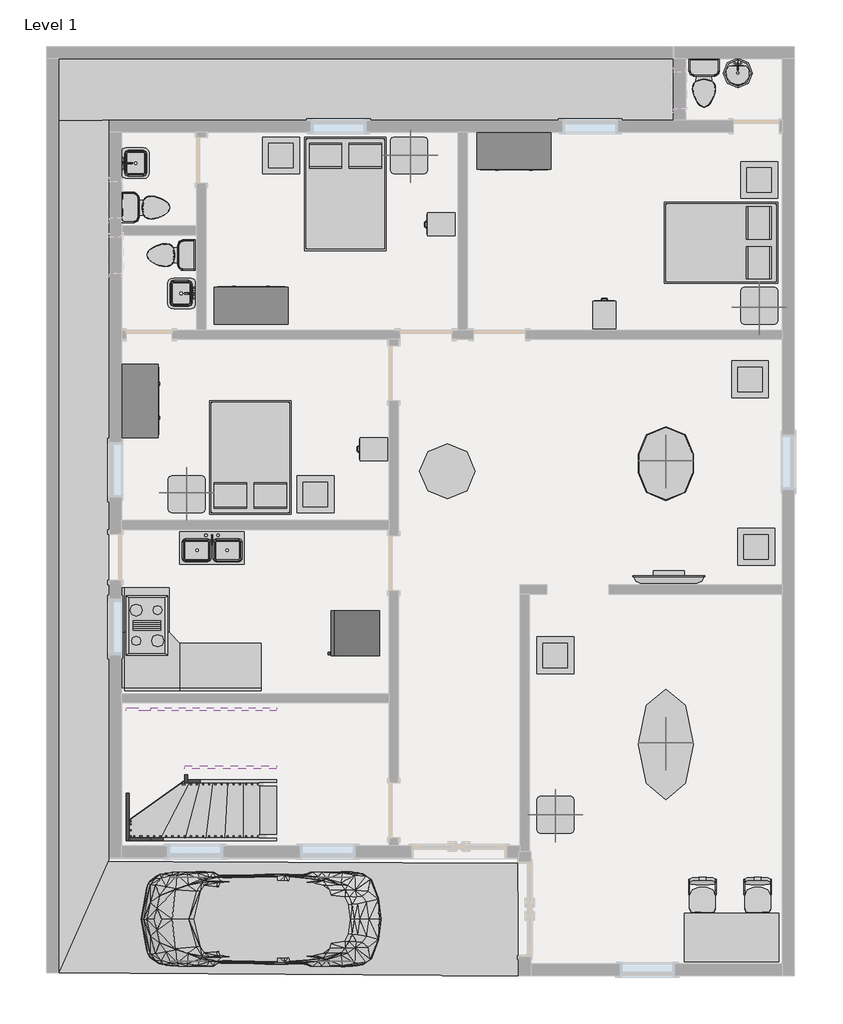
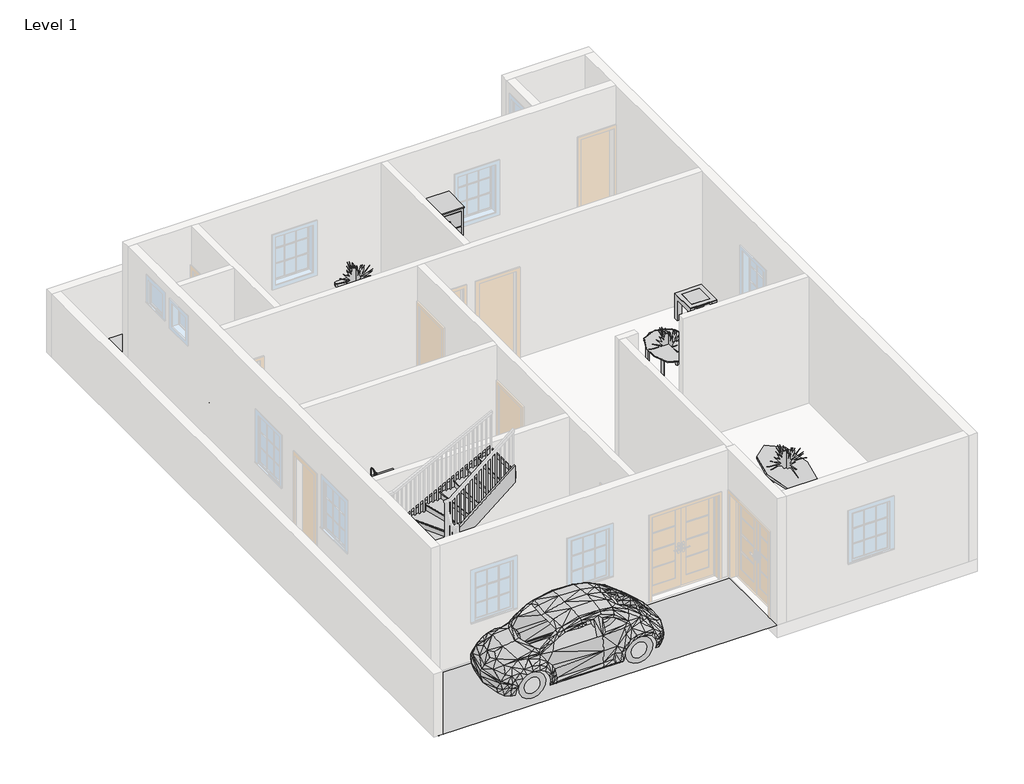
# One storey, part 3 of 3: 27 furniture elements, 10 flow terminals, 8 members, 6 geographic elements, 6 proxies, 1 stair flight.
"""IFC4 building model written with IfcOpenShell, lengths in millimetres."""

from ifc_helpers import new_model, si_unit, frame, origin, place, context, project, spatial, polyline, outline, extrude, triangles, transform, mapped, element, save
from components import proxy_bb1e6e30, rpc_beetle_rpc_beetle_3ce7ba48, proxy_a13a33b2, flow_terminal_accce45a, flow_terminal_a53be723, flow_terminal_d49f872f, flow_terminal_62a433f7, toilet_domestic_3d_toilet_domestic_3d_f7549cf7, toilet_domestic_3d_toilet_domestic_3d_183bbd19, furniture_c8abb964, furniture_bb55ed6b, furniture_072f6425, furniture_9fa109b2, furniture_3d1d9cbc, furniture_d9bcc661, furniture_b5c51a22, furniture_be1c6672, furniture_905aceb5, furniture_c0716227, furniture_31d08a24, furniture_cb58875c, rpc_plant_tropical_agave_1_5_93a2a214, stair_flight_2afbddc8

model = new_model("IFC4")

# Units and contexts
model_context = context("Model", 3, world=origin())
ifc_project = project(units=[si_unit("LENGTHUNIT", "METRE", prefix="MILLI")], contexts=[model_context])

# Site, building, storey
site = spatial("IfcSite", under=ifc_project)
building = spatial("IfcBuilding", under=site)
storey = spatial("IfcBuildingStorey", under=building, Name="Level 1", Elevation=0.0)

# Proxies
placement = place(None, origin())
element("IfcBuildingElementProxy", 1, Name="Building Element Proxy", at=placement, inside=storey, context=model_context, shape_type="Tessellation", body=[
    triangles([(813.744298, 15274.0246674, 0.0), (801.0442738, 14258.0250549, 0.0), (-9384.3556778, 14243.023645, 0.0), (-9384.3556778, 15274.0246674, 0.0)], [[4, 3, 2], [2, 1, 4]], closed=False),
])
element("IfcBuildingElementProxy", 2, Name="Building Element Proxy", at=placement, inside=storey, context=model_context, shape_type="Tessellation", body=[
    triangles([(-8546.1556778, 14258.0250549, 0.0), (-9384.3556778, 14196.8846008, 0.0), (-9384.3556778, 135.6245977, 0.0), (-9384.3556778, 2055.4156734, 0.0), (-8546.1556778, 2021.5745705, 0.0), (-9384.3556778, 14248.2919281, 0.0)], [[5, 4, 3], [5, 2, 4], [6, 2, 1], [5, 1, 2]], closed=False),
])
element("IfcBuildingElementProxy", 3, Name="Building Element Proxy", at=placement, inside=storey, context=model_context, shape_type="Tessellation", body=[
    triangles([(-9384.3556778, 1984.3604176, 0.0), (-1783.4056778, 1951.7246189, 0.0), (-1764.3556778, 84.8246007, 0.0), (-9485.9558716, 135.6245977, 0.0), (-9384.3556778, 135.6245977, 0.0)], [[1, 4, 5], [5, 3, 2], [3, 5, 4], [5, 2, 1]], closed=False),
])
proxy_shape = proxy_bb1e6e30(model_context)
element("IfcBuildingElementProxy", 4, Name="Cook Top-4 Unit : 36\" x 20\"", ObjectType="Cook Top-4 Unit : 36\" x 20\"", at=placement, inside=storey, context=model_context, shape_type="MappedRepresentation", body=[
    mapped(proxy_shape, transform((-7923.8557202, 5888.7245992, 0.0), x_axis=(0.0, 1.0000000000000002, 0.0), y_axis=(-1.0000000000000002, 0.0, 0.0), z_axis=(0.0, 0.0, 1.0))),
])
rpc_beetle_rpc_beetle_shape = rpc_beetle_rpc_beetle_3ce7ba48(model_context)
element("IfcBuildingElementProxy", 5, Name="RPC Beetle : RPC Beetle", ObjectType="RPC Beetle : RPC Beetle", at=placement, inside=storey, context=model_context, shape_type="MappedRepresentation", body=[
    mapped(rpc_beetle_rpc_beetle_shape, transform((-4799.6557202, 1024.6245992, 0.0), x_axis=(0.0, 1.0000000000000002, 0.0), y_axis=(-1.0000000000000002, 0.0, 0.0), z_axis=(0.0, 0.0, 1.0))),
])
proxy_2_shape = proxy_a13a33b2(model_context)
element("IfcBuildingElementProxy", 6, Name="Refrigerator : 30\" x 32\" RH", ObjectType="Refrigerator : 30\" x 32\" RH", at=placement, inside=storey, context=model_context, shape_type="MappedRepresentation", body=[
    mapped(proxy_2_shape, transform((-4455.5567488, 5756.9620992, 0.0), x_axis=(0.0, -1.0000000000000007, 0.0), y_axis=(1.0000000000000007, 0.0, 0.0), z_axis=(0.0, 0.0, 1.0))),
])

# Flow terminals
flow_terminal_shape = flow_terminal_accce45a(model_context)
element("IfcFlowTerminal", 7, ObjectType="Floor Drain - Round : 5\" Strainer - 2\" Drain", at=placement, inside=storey, context=model_context, shape_type="MappedRepresentation", body=[
    mapped(flow_terminal_shape, transform((-7276.1557202, 12937.2245992, 0.0), x_axis=(1.0, 0.0, 0.0), y_axis=(0.0, 1.0, 0.0), z_axis=(0.0, 0.0, 1.0))),
])
element("IfcFlowTerminal", 8, ObjectType="Floor Drain - Round : 5\" Strainer - 2\" Drain", at=placement, inside=storey, context=model_context, shape_type="MappedRepresentation", body=[
    mapped(flow_terminal_shape, transform((-8101.6557202, 11743.4245992, 0.0), x_axis=(1.0, 0.0, 0.0), y_axis=(0.0, 1.0, 0.0), z_axis=(0.0, 0.0, 1.0))),
])
element("IfcFlowTerminal", 9, ObjectType="Floor Drain - Round : 5\" Strainer - 2\" Drain", at=placement, inside=storey, context=model_context, shape_type="MappedRepresentation", body=[
    mapped(flow_terminal_shape, transform((1537.6442798, 14410.4245992, 0.0), x_axis=(1.0, 0.0, 0.0), y_axis=(0.0, 1.0, 0.0), z_axis=(0.0, 0.0, 1.0))),
])
flow_terminal_2_shape = flow_terminal_a53be723(model_context)
element("IfcFlowTerminal", 10, ObjectType="Sink Kitchen-Double : 42\" x 21\"", at=placement, inside=storey, context=model_context, shape_type="MappedRepresentation", body=[
    mapped(flow_terminal_2_shape, transform((-6860.0449608, 7169.0791981, 0.0), x_axis=(1.0, 0.0, 0.0), y_axis=(0.0, 1.0, 0.0), z_axis=(0.0, 0.0, 1.0))),
])
flow_terminal_3_shape = flow_terminal_d49f872f(model_context)
element("IfcFlowTerminal", 11, ObjectType="Sink Vanity-Round : 19\" x 19\"", at=placement, inside=storey, context=model_context, shape_type="MappedRepresentation", body=[
    mapped(flow_terminal_3_shape, transform((1771.1925392, 14953.8924693, 0.0), x_axis=(1.0, 0.0, 0.0), y_axis=(0.0, 1.0, 0.0), z_axis=(0.0, 0.0, 1.0))),
])
flow_terminal_4_shape = flow_terminal_62a433f7(model_context)
element("IfcFlowTerminal", 12, ObjectType="Sink Vanity-Square : 20\" x 18\"", at=placement, inside=storey, context=model_context, shape_type="MappedRepresentation", body=[
    mapped(flow_terminal_4_shape, transform((-8162.8103191, 13531.1353587, 0.0), x_axis=(0.0, 1.0000000000000002, 0.0), y_axis=(-1.0000000000000002, 0.0, 0.0), z_axis=(0.0, 0.0, 1.0))),
])
element("IfcFlowTerminal", 13, ObjectType="Sink Vanity-Square : 20\" x 18\"", at=placement, inside=storey, context=model_context, shape_type="MappedRepresentation", body=[
    mapped(flow_terminal_4_shape, transform((-7303.9011214, 11403.5138398, 0.0), x_axis=(0.0, -1.0000000000000004, 0.0), y_axis=(1.0000000000000004, 0.0, 0.0), z_axis=(0.0, 0.0, 1.0))),
])
toilet_domestic_3d_toilet_domestic_3d_shape = toilet_domestic_3d_toilet_domestic_3d_f7549cf7(model_context)
toilet_domestic_3d_toilet_domestic_3d_2_shape = toilet_domestic_3d_toilet_domestic_3d_183bbd19(model_context)
element("IfcFlowTerminal", 14, ObjectType="Toilet-Domestic-3D : Toilet-Domestic-3D", at=placement, inside=storey, context=model_context, shape_type="MappedRepresentation", body=[
    mapped(toilet_domestic_3d_toilet_domestic_3d_shape, transform((-7848.2596929, 12810.2245992, 0.0), x_axis=(0.0, 1.0000000000000002, 0.0), y_axis=(-1.0000000000000002, 0.0, 0.0), z_axis=(0.0, 0.0, 1.0))),
    mapped(toilet_domestic_3d_toilet_domestic_3d_2_shape, transform((-7848.2596929, 12810.2245992, 0.0), x_axis=(0.0, 1.0000000000000002, 0.0), y_axis=(-1.0000000000000002, 0.0, 0.0), z_axis=(0.0, 0.0, 1.0))),
])
element("IfcFlowTerminal", 15, ObjectType="Toilet-Domestic-3D : Toilet-Domestic-3D", at=placement, inside=storey, context=model_context, shape_type="MappedRepresentation", body=[
    mapped(toilet_domestic_3d_toilet_domestic_3d_shape, transform((-7618.4517476, 12022.8245992, 0.0), x_axis=(0.0, -1.0000000000000002, 0.0), y_axis=(1.0000000000000002, 0.0, 0.0), z_axis=(0.0, 0.0, 1.0))),
    mapped(toilet_domestic_3d_toilet_domestic_3d_2_shape, transform((-7618.4517476, 12022.8245992, 0.0), x_axis=(0.0, -1.0000000000000002, 0.0), y_axis=(1.0000000000000002, 0.0, 0.0), z_axis=(0.0, 0.0, 1.0))),
])
element("IfcFlowTerminal", 16, ObjectType="Toilet-Domestic-3D : Toilet-Domestic-3D", at=placement, inside=storey, context=model_context, shape_type="MappedRepresentation", body=[
    mapped(toilet_domestic_3d_toilet_domestic_3d_shape, transform((1309.0442798, 14779.3285719, 0.0), x_axis=(1.0000000000000002, 0.0, 0.0), y_axis=(0.0, 1.0000000000000002, 0.0), z_axis=(0.0, 0.0, 1.0))),
    mapped(toilet_domestic_3d_toilet_domestic_3d_2_shape, transform((1309.0442798, 14779.3285719, 0.0), x_axis=(1.0000000000000002, 0.0, 0.0), y_axis=(0.0, 1.0000000000000002, 0.0), z_axis=(0.0, 0.0, 1.0))),
])

# Furniture
furniture_shape = furniture_c8abb964(model_context)
element("IfcFurniture", 17, ObjectType="Bed-Box : Double 53\" x 74\"", at=placement, inside=storey, context=model_context, shape_type="MappedRepresentation", body=[
    mapped(furniture_shape, transform((-4973.7081793, 13273.2541074, 0.0), x_axis=(1.0, 0.0, 0.0), y_axis=(0.0, 1.0, 0.0), z_axis=(0.0, 0.0, 1.0))),
])
element("IfcFurniture", 18, ObjectType="Bed-Box : Double 53\" x 74\"", at=placement, inside=storey, context=model_context, shape_type="MappedRepresentation", body=[
    mapped(furniture_shape, transform((1822.873788, 12565.1770582, 0.0), x_axis=(0.0, -1.0000000000000002, 0.0), y_axis=(1.0000000000000002, 0.0, 0.0), z_axis=(0.0, 0.0, 1.0))),
])
element("IfcFurniture", 19, ObjectType="Bed-Box : Double 53\" x 74\"", at=placement, inside=storey, context=model_context, shape_type="MappedRepresentation", body=[
    mapped(furniture_shape, transform((-5870.2032612, 8435.595091, 0.0), x_axis=(-1.0000000000000002, 0.0, 0.0), y_axis=(0.0, -1.0000000000000002, 0.0), z_axis=(0.0, 0.0, 1.0))),
])
furniture_2_shape = furniture_bb55ed6b(model_context)
element("IfcFurniture", 20, ObjectType="Cabinet-File 2 Drawer : 15\" x 18\"", at=placement, inside=storey, context=model_context, shape_type="MappedRepresentation", body=[
    mapped(furniture_2_shape, transform((-2904.9214201, 12402.9281522, 0.0), x_axis=(0.0, -1.0000000000000002, 0.0), y_axis=(1.0000000000000002, 0.0, 0.0), z_axis=(0.0, 0.0, 1.0))),
])
element("IfcFurniture", 21, ObjectType="Cabinet-File 2 Drawer : 15\" x 18\"", at=placement, inside=storey, context=model_context, shape_type="MappedRepresentation", body=[
    mapped(furniture_2_shape, transform((-469.8521673, 10890.0902991, 0.0), x_axis=(-0.9999999999999998, 0.0, 0.0), y_axis=(0.0, -0.9999999999999998, 0.0), z_axis=(0.0, 0.0, 1.0))),
])
element("IfcFurniture", 22, ObjectType="Cabinet-File 2 Drawer : 15\" x 18\"", at=placement, inside=storey, context=model_context, shape_type="MappedRepresentation", body=[
    mapped(furniture_2_shape, transform((-4022.5214201, 8681.8281522, 0.0), x_axis=(0.0, -1.0000000000000002, 0.0), y_axis=(1.0000000000000002, 0.0, 0.0), z_axis=(0.0, 0.0, 1.0))),
])
furniture_3_shape = furniture_072f6425(model_context)
element("IfcFurniture", 23, ObjectType="Desk : 60\" x 30\" Student", at=placement, inside=storey, context=model_context, shape_type="MappedRepresentation", body=[
    mapped(furniture_3_shape, transform((1004.2442798, 338.8245992, 0.0), x_axis=(1.0000000000000004, 0.0, 0.0), y_axis=(0.0, 1.0000000000000004, 0.0), z_axis=(0.0, 0.0, 1.0))),
])
furniture_4_shape = furniture_9fa109b2(model_context)
element("IfcFurniture", 24, ObjectType="Dresser : 48\" x 72\" x 24\"", at=placement, inside=storey, context=model_context, shape_type="MappedRepresentation", body=[
    mapped(furniture_4_shape, transform((-6465.8489801, 10821.4616451, 0.0), x_axis=(-1.0000000000000004, 0.0, 0.0), y_axis=(0.0, -1.0000000000000004, 0.0), z_axis=(0.0, 0.0, 1.0))),
])
element("IfcFurniture", 25, ObjectType="Dresser : 48\" x 72\" x 24\"", at=placement, inside=storey, context=model_context, shape_type="MappedRepresentation", body=[
    mapped(furniture_4_shape, transform((-1571.3624604, 14113.1875533, 0.0), x_axis=(1.0, 0.0, 0.0), y_axis=(0.0, 1.0, 0.0), z_axis=(0.0, 0.0, 1.0))),
])
element("IfcFurniture", 26, ObjectType="Dresser : 48\" x 72\" x 24\"", at=placement, inside=storey, context=model_context, shape_type="MappedRepresentation", body=[
    mapped(furniture_4_shape, transform((-8401.3186743, 9879.0178591, 0.0), x_axis=(0.0, 1.0000000000000002, 0.0), y_axis=(-1.0000000000000002, 0.0, 0.0), z_axis=(0.0, 0.0, 1.0))),
])
furniture_5_shape = furniture_3d1d9cbc(model_context)
element("IfcFurniture", 27, ObjectType="Seating-Auditorium : 18\" x 24\" x 30\"", at=placement, inside=storey, context=model_context, shape_type="MappedRepresentation", body=[
    mapped(furniture_5_shape, transform((2358.7721486, 1620.9000091, 0.0), x_axis=(-1.0000000000000004, 0.0, 0.0), y_axis=(0.0, -1.0000000000000004, 0.0), z_axis=(0.0, 0.0, 1.0))),
])
element("IfcFurniture", 28, ObjectType="Seating-Auditorium : 18\" x 24\" x 30\"", at=placement, inside=storey, context=model_context, shape_type="MappedRepresentation", body=[
    mapped(furniture_5_shape, transform((1444.3721486, 1620.9000091, 0.0), x_axis=(-1.0, 0.0, 0.0), y_axis=(0.0, -1.0, 0.0), z_axis=(0.0, 0.0, 1.0))),
])
furniture_6_shape = furniture_d9bcc661(model_context)
element("IfcFurniture", 29, ObjectType="TV - Flat Screen : 46\"", at=placement, inside=storey, context=model_context, shape_type="MappedRepresentation", body=[
    mapped(furniture_6_shape, transform((720.8997656, 6645.7632229, 0.0), x_axis=(-1.0, 0.0, 0.0), y_axis=(0.0, -1.0, 0.0), z_axis=(0.0, 0.0, 1.0))),
])
furniture_7_shape = furniture_b5c51a22(model_context)
element("IfcFurniture", 30, ObjectType="Table-Coffee : 24\" x 24\" x 24\"", at=placement, inside=storey, context=model_context, shape_type="MappedRepresentation", body=[
    mapped(furniture_7_shape, transform((-5719.6214869, 13578.6135214, 0.0), x_axis=(1.0, 0.0, 0.0), y_axis=(0.0, 1.0, 0.0), z_axis=(0.0, 0.0, 1.0))),
])
element("IfcFurniture", 31, ObjectType="Table-Coffee : 24\" x 24\" x 24\"", at=placement, inside=storey, context=model_context, shape_type="MappedRepresentation", body=[
    mapped(furniture_7_shape, transform((2205.1785131, 13172.2135214, 0.0), x_axis=(1.0, 0.0, 0.0), y_axis=(0.0, 1.0, 0.0), z_axis=(0.0, 0.0, 1.0))),
])
element("IfcFurniture", 32, ObjectType="Table-Coffee : 24\" x 24\" x 24\"", at=placement, inside=storey, context=model_context, shape_type="MappedRepresentation", body=[
    mapped(furniture_7_shape, transform((-5148.1214869, 7965.2135214, 0.0), x_axis=(1.0, 0.0, 0.0), y_axis=(0.0, 1.0, 0.0), z_axis=(0.0, 0.0, 1.0))),
])
element("IfcFurniture", 33, ObjectType="Table-Coffee : 24\" x 24\" x 24\"", at=placement, inside=storey, context=model_context, shape_type="MappedRepresentation", body=[
    mapped(furniture_7_shape, transform((2052.7785131, 9870.2135214, 0.0), x_axis=(1.0, 0.0, 0.0), y_axis=(0.0, 1.0, 0.0), z_axis=(0.0, 0.0, 1.0))),
])
element("IfcFurniture", 34, ObjectType="Table-Coffee : 24\" x 24\" x 24\"", at=placement, inside=storey, context=model_context, shape_type="MappedRepresentation", body=[
    mapped(furniture_7_shape, transform((2154.3785131, 7095.2635214, 0.0), x_axis=(1.0, 0.0, 0.0), y_axis=(0.0, 1.0, 0.0), z_axis=(0.0, 0.0, 1.0))),
])
element("IfcFurniture", 35, ObjectType="Table-Coffee : 24\" x 24\" x 24\"", at=placement, inside=storey, context=model_context, shape_type="MappedRepresentation", body=[
    mapped(furniture_7_shape, transform((-1173.0214869, 5298.2135214, 0.0), x_axis=(1.0, 0.0, 0.0), y_axis=(0.0, 1.0, 0.0), z_axis=(0.0, 0.0, 1.0))),
])
furniture_8_shape = furniture_be1c6672(model_context)
element("IfcFurniture", 36, ObjectType="Table-Dining Oval : 36\" x 48\"", at=placement, inside=storey, context=model_context, shape_type="MappedRepresentation", body=[
    mapped(furniture_8_shape, transform((315.9459191, 8970.2442714, 0.0), x_axis=(0.0, 1.0, 0.0), y_axis=(-1.0, 0.0, 0.0), z_axis=(0.0, 0.0, 1.0))),
])
furniture_9_shape = furniture_905aceb5(model_context)
element("IfcFurniture", 37, ObjectType="Table-Dining Round w Chairs : 36\" Diameter", at=placement, inside=storey, context=model_context, shape_type="MappedRepresentation", body=[
    mapped(furniture_9_shape, transform((-3049.1376875, 8626.3032878, 0.0), x_axis=(1.0, 0.0, 0.0), y_axis=(0.0, 1.0, 0.0), z_axis=(0.0, 0.0, 1.0))),
])
furniture_10_shape = furniture_c0716227(model_context)
element("IfcFurniture", 38, ObjectType="Table-Ellipse : 72\" x 36\"", at=placement, inside=storey, context=model_context, shape_type="MappedRepresentation", body=[
    mapped(furniture_10_shape, transform((674.0442798, 3920.2245992, 0.0), x_axis=(0.0, 1.0, 0.0), y_axis=(-1.0, 0.0, 0.0), z_axis=(0.0, 0.0, 1.0))),
])
furniture_11_shape = furniture_31d08a24(model_context)
element("IfcFurniture", 39, ObjectType="Table-End : 24\" x 24\"", at=placement, inside=storey, context=model_context, shape_type="MappedRepresentation", body=[
    mapped(furniture_11_shape, transform((-3888.9893505, 13521.4245992, 0.0), x_axis=(1.0, 0.0, 0.0), y_axis=(0.0, 1.0, 0.0), z_axis=(0.0, 0.0, 1.0))),
])
element("IfcFurniture", 40, ObjectType="Table-End : 24\" x 24\"", at=placement, inside=storey, context=model_context, shape_type="MappedRepresentation", body=[
    mapped(furniture_11_shape, transform((1914.9106495, 11032.2245992, 0.0), x_axis=(1.0, 0.0, 0.0), y_axis=(0.0, 1.0, 0.0), z_axis=(0.0, 0.0, 1.0))),
])
element("IfcFurniture", 41, ObjectType="Table-End : 24\" x 24\"", at=placement, inside=storey, context=model_context, shape_type="MappedRepresentation", body=[
    mapped(furniture_11_shape, transform((-7571.9893505, 7908.0245992, 0.0), x_axis=(1.0, 0.0, 0.0), y_axis=(0.0, 1.0, 0.0), z_axis=(0.0, 0.0, 1.0))),
])
element("IfcFurniture", 42, ObjectType="Table-End : 24\" x 24\"", at=placement, inside=storey, context=model_context, shape_type="MappedRepresentation", body=[
    mapped(furniture_11_shape, transform((-1463.2893505, 2599.4245992, 0.0), x_axis=(1.0, 0.0, 0.0), y_axis=(0.0, 1.0, 0.0), z_axis=(0.0, 0.0, 1.0))),
])
furniture_12_shape = furniture_cb58875c(model_context)
element("IfcFurniture", 43, ObjectType="Work Station Cubicle : 96\" x 96\"", at=placement, inside=storey, context=model_context, shape_type="MappedRepresentation", body=[
    mapped(furniture_12_shape, transform((-8837.9787279, 4940.9563515, 0.0), x_axis=(0.0, 1.0000000000000002, 0.0), y_axis=(-1.0000000000000002, 0.0, 0.0), z_axis=(0.0, 0.0, 1.0))),
])

# Geographic elements
rpc_plant_tropical_agave_1_5_shape = rpc_plant_tropical_agave_1_5_93a2a214(model_context)
element("IfcGeographicElement", 44, ObjectType="RPC Plant - Tropical : Agave - 1.5'", at=placement, inside=storey, context=model_context, shape_type="MappedRepresentation", body=[
    mapped(rpc_plant_tropical_agave_1_5_shape, transform((-3555.0557202, 13673.8245992, 609.6), x_axis=(1.0, 0.0, 0.0), y_axis=(0.0, 1.0, 0.0), z_axis=(0.0, 0.0, 1.0))),
])
element("IfcGeographicElement", 45, ObjectType="RPC Plant - Tropical : Agave - 1.5'", at=placement, inside=storey, context=model_context, shape_type="MappedRepresentation", body=[
    mapped(rpc_plant_tropical_agave_1_5_shape, transform((2223.4442798, 11159.2245992, 609.6), x_axis=(1.0, 0.0, 0.0), y_axis=(0.0, 1.0, 0.0), z_axis=(0.0, 0.0, 1.0))),
])
element("IfcGeographicElement", 46, ObjectType="RPC Plant - Tropical : Agave - 1.5'", at=placement, inside=storey, context=model_context, shape_type="MappedRepresentation", body=[
    mapped(rpc_plant_tropical_agave_1_5_shape, transform((-7263.4557202, 8085.8245992, 609.6), x_axis=(1.0, 0.0, 0.0), y_axis=(0.0, 1.0, 0.0), z_axis=(0.0, 0.0, 1.0))),
])
element("IfcGeographicElement", 47, ObjectType="RPC Plant - Tropical : Agave - 1.5'", at=placement, inside=storey, context=model_context, shape_type="MappedRepresentation", body=[
    mapped(rpc_plant_tropical_agave_1_5_shape, transform((674.0442798, 8619.2245992, 609.6), x_axis=(1.0, 0.0, 0.0), y_axis=(0.0, 1.0, 0.0), z_axis=(0.0, 0.0, 1.0))),
])
element("IfcGeographicElement", 48, ObjectType="RPC Plant - Tropical : Agave - 1.5'", at=placement, inside=storey, context=model_context, shape_type="MappedRepresentation", body=[
    mapped(rpc_plant_tropical_agave_1_5_shape, transform((674.0442798, 3945.6245992, 609.6), x_axis=(1.0, 0.0, 0.0), y_axis=(0.0, 1.0, 0.0), z_axis=(0.0, 0.0, 1.0))),
])
element("IfcGeographicElement", 49, ObjectType="RPC Plant - Tropical : Agave - 1.5'", at=placement, inside=storey, context=model_context, shape_type="MappedRepresentation", body=[
    mapped(rpc_plant_tropical_agave_1_5_shape, transform((-1154.7557202, 2751.8245992, 609.6), x_axis=(1.0, 0.0, 0.0), y_axis=(0.0, 1.0, 0.0), z_axis=(0.0, 0.0, 1.0))),
])

# Members
element("IfcMember", 50, ObjectType="Stringer - 2\" Width", at=placement, inside=storey, context=model_context, shape_type="SweptSolid", body=[
    extrude(outline(polyline([(0.0, -5773.8240284), (229.639954, -5773.8240284), (1305.3956453, -7861.2412201), (962.500629, -7861.2412201), (0.0, -5993.5863459), (0.0, -5773.8240284)])), frame((0.0, 2320.0245992, 0.0), z_axis=(0.0, 1.0, 0.0), x_axis=(0.0, 0.0, 1.0)), (0.0, 0.0, 1.0), 50.8),
])
element("IfcMember", 51, ObjectType="Stringer - 2\" Width", at=placement, inside=storey, context=model_context, shape_type="SweptSolid", body=[
    extrude(outline(polyline([(-7861.2412201, 2370.8245992), (-7861.2412201, 2320.0245992), (-8215.9557202, 2320.0245992), (-8215.9557202, 2370.8245992), (-7861.2412201, 2370.8245992)])), frame((0.0, 0.0, 962.500629), z_axis=(0.0, 0.0, 1.0), x_axis=(1.0, 0.0, 0.0)), (0.0, 0.0, 1.0), 342.8950162),
])
element("IfcMember", 52, ObjectType="Stringer - 2\" Width", at=placement, inside=storey, context=model_context, shape_type="SweptSolid", body=[
    extrude(outline(polyline([(2320.0245992, 1000.5956453), (2320.0245992, 1289.0952212), (4442.0444819, 1969.9972697), (4479.0245992, 1969.9972697), (4479.0245992, 1638.9682298), (2489.5470822, 1000.5956453), (2320.0245992, 1000.5956453)])), frame((-8266.7557202, 0.0, 0.0), z_axis=(1.0, 0.0, 0.0), x_axis=(0.0, 1.0, 0.0)), (0.0, 0.0, 1.0), 50.8),
])
element("IfcMember", 53, ObjectType="Stringer - 2\" Width", at=placement, inside=storey, context=model_context, shape_type="SweptSolid", body=[
    extrude(outline(polyline([(-8266.7557202, 4479.0245992), (-8266.7557202, 4529.8245992), (-7861.2412201, 4529.8245992), (-7861.2412201, 4479.0245992), (-8266.7557202, 4479.0245992)])), frame((0.0, 0.0, 1649.8904473), z_axis=(0.0, 0.0, 1.0), x_axis=(1.0, 0.0, 0.0)), (0.0, 0.0, 1.0), 320.1068224),
])
element("IfcMember", 54, ObjectType="Stringer - 2\" Width", at=placement, inside=storey, context=model_context, shape_type="SweptSolid", body=[
    extrude(outline(polyline([(1969.9972697, -7861.2412201), (1649.8904473, -7861.2412201), (2725.6461385, -5773.8240284), (3045.7529609, -5773.8240284), (1969.9972697, -7861.2412201)])), frame((0.0, 4479.0245992, 0.0), z_axis=(0.0, 1.0, 0.0), x_axis=(0.0, 0.0, 1.0)), (0.0, 0.0, 1.0), 50.8),
])
element("IfcMember", 55, ObjectType="Stringer - 2\" Width", at=placement, inside=storey, context=model_context, shape_type="SweptSolid", body=[
    extrude(outline(polyline([(0.0, -5773.8240284), (176.1764461, -5773.8240284), (1380.418648, -7250.7557202), (987.1410923, -7250.7557202), (0.0, -6040.0856729), (0.0, -5773.8240284)])), frame((0.0, 3285.2245992, 0.0), z_axis=(0.0, 1.0, 0.0), x_axis=(0.0, 0.0, 1.0)), (0.0, 0.0, 1.0), 50.8),
])
element("IfcMember", 56, ObjectType="Stringer - 2\" Width", at=placement, inside=storey, context=model_context, shape_type="SweptSolid", body=[
    extrude(outline(polyline([(3285.2245992, 1028.5617647), (3285.2245992, 1573.2682978), (3491.8617167, 1926.1409689), (3513.8245992, 1926.1409689), (3513.8245992, 1360.465107), (3319.4668165, 1028.5617647), (3285.2245992, 1028.5617647)])), frame((-7301.5557202, 0.0, 0.0), z_axis=(1.0, 0.0, 0.0), x_axis=(0.0, 1.0, 0.0)), (0.0, 0.0, 1.0), 50.8),
])
element("IfcMember", 57, ObjectType="Stringer - 2\" Width", at=placement, inside=storey, context=model_context, shape_type="SweptSolid", body=[
    extrude(outline(polyline([(1926.1409689, -7301.5557202), (1532.8634131, -7301.5557202), (2778.5262875, -5773.8240284), (3171.8038432, -5773.8240284), (1926.1409689, -7301.5557202)])), frame((0.0, 3513.8245992, 0.0), z_axis=(0.0, 1.0, 0.0), x_axis=(0.0, 0.0, 1.0)), (0.0, 0.0, 1.0), 50.8),
])

# Stair flight
stair_flight_shape = stair_flight_2afbddc8(model_context)
element("IfcStairFlight", 58, ObjectType="2\" Tread 1\" Nosing 1/4\" Riser", at=placement, inside=storey, context=model_context, shape_type="MappedRepresentation", body=[
    mapped(stair_flight_shape, transform((0.0, 0.0, 0.0), x_axis=(1.0, 0.0, 0.0), y_axis=(0.0, 1.0, 0.0), z_axis=(0.0, 0.0, 1.0))),
])

save(model, "model.ifc")

# Revit data of these elements
# Type "Cook Top-4 Unit : 36\" x 20\""
#   Assembly Code = "E1090400"
#   Depth = 2' - 0"
#   Width = 3' - 0"
#   Burner Material = Steel, Chrome Plated
#   Cooktop Material = Steel, Polished
#   Default Elevation = 0
# Type "RPC Beetle : RPC Beetle"
#   built-in parameter 1005195 = "RPC-16-0U6E-L4EG-ENH1-J3KF-SVEL-0TX4-C0"
#   Height = 0
# Type "Refrigerator : 30\" x 32\" RH"
#   Label = "REF."
#   Assembly Code = "E1090400"
#   Depth = 2' - 7 3/4"
#   Handle = 2' - 3"
#   Height = 5' - 10"
#   Rear Clearance = 0' - 2"
#   Top Door Height = 1' - 8"
#   Width = 2' - 5 3/8"
#   Material = Steel, Paint Finish, Ivory, Glossy
#   Default Elevation = 0
# Type "Floor Drain - Round : 5\" Strainer - 2\" Drain"
#   WFU = 2
#   Strainer Height = 0' - 3 1/4"
#   Strainer Radius = 0' - 2 1/2"
#   Strainer Diameter = 0' - 5"
#   Radius 6 = 0' - 0 5/8"
#   Radius 5 = 0' - 1 1/4"
#   Radius 4 = 0' - 1 7/8"
#   Radius 2 = 0' - 3.04167"
#   Radius 1 = 0' - 2.02083"
#   Radius 3 = 0' - 2 1/32"
#   Pipe Radius = 1"
#   Pipe Diameter = 2"
#   Height 2 = 0' - 0.725"
#   Height 1 = 0' - 1 13/16"
#   Body Radius = 0' - 4 1/16"
#   Body Height = 0' - 3 5/8"
#   Body Diameter = 0' - 8 1/8"
#   Drain Material = none
#   HWFU = 0
#   Default Elevation = 0
#   CWFU = 0
# Type "Sink Kitchen-Double : 42\" x 21\""
#   Assembly Code = "D2010410"
#   Counter Height = 3' - 0"
#   Depth = 1' - 9"
#   Width = 3' - 6"
#   Faucet Material = Steel, Polished
#   Sink Material = Steel, Polished
#   Default Elevation = 0
# Type "Sink Vanity-Round : 19\" x 19\""
#   Assembly Code = "D2010400"
#   Top Of Counter = 2' - 7"
#   Basin Material = Porcelain, Linen
#   Faucet Material = Steel, Polished
#   Default Elevation = 0
# Type "Sink Vanity-Square : 20\" x 18\""
#   Assembly Code = "D2010400"
#   Counter Height = 2' - 7"
#   Depth = 1' - 6"
#   Width = 1' - 8"
#   Basin Material = Porcelain, Linen
#   Faucet Material = Steel, Polished
#   Default Elevation = 0
# Type "Toilet-Domestic-3D : Toilet-Domestic-3D"
#   Assembly Code = "D2010110"
#   Toilet - Bowl/Basin Material = Porcelain, Linen
#   Toilet - Seat Material = Laminate, Linen, Matte
#   Default Elevation = 0
# Type "Bed-Box : Double 53\" x 74\""
#   Assembly Code = "E2020200"
#   Length = 6' - 2"
#   Width = 4' - 5"
#   Frame Material = Birch
#   Mattress Material = Linen, White
#   Default Elevation = 0
# Type "Cabinet-File 2 Drawer : 15\" x 18\""
#   Assembly Code = "E2020200"
#   Depth = 1' - 6"
#   Height = 2' - 5"
#   Width = 1' - 3"
#   Cabinet Material = Steel, Paint Finish, Ivory, Glossy
#   Handle Material = Steel, Chrome Plated
#   Default Elevation = 0
# Type "Desk : 60\" x 30\" Student"
#   Assembly Code = "E2020200"
#   Depth = 2' - 6"
#   Height = 2' - 6"
#   Leg Height = 0' - 6"
#   Width = 5' - 0"
#   Body Material = Laminate, Ivory, Matte
#   Handle/Leg Material = Steel, Chrome Plated
#   Top Material = Cherry
#   Default Elevation = 0
# Type "Dresser : 48\" x 72\" x 24\""
#   Assembly Code = "E2020200"
#   Depth = 2' - 0"
#   Height = 6' - 0"
#   Width = 4' - 0"
#   Dresser Material = Laminate - Ivory, Glossy
#   Drawer Material = Laminate, Ivory, Matte
#   Knob Material = Cherry
#   Default Elevation = 0
# Type "Seating-Auditorium : 18\" x 24\" x 30\""
#   Assembly Code = "E2020200"
#   Seat Material = Linen, Beige
#   Frame Material = Steel, Paint Finish, Dark Gray, Matte
#   Default Elevation = 0
# Type "TV - Flat Screen : 46\""
#   SinAng = 0' - 0.0193"
#   L = 3' - 4.83276"
#   H = 1' - 10.97053"
#   Thickness = 0' - 4.33071"
#   Diagonal = 3' - 10.85039"
#   CosAng = 0' - 0.03431"
#   Stand [instance default] = yes
#   Default Elevation = 0
# Type "Table-Coffee : 24\" x 24\" x 24\""
#   Assembly Code = "E2020200"
#   Height = 2' - 0"
#   Length = 2' - 0"
#   Width = 2' - 0"
#   Top Material = none
#   Frame Material = none
#   Default Elevation = 0
# Type "Table-Dining Oval : 36\" x 48\""
#   Assembly Code = "E2020200"
#   Length = 4' - 0"
#   Width = 3' - 0"
#   Base Material = Steel, Chrome Plated
#   Top Material = Glass - Clear, Grey
#   Default Elevation = 0
#   Description = (empty or 0)
# Type "Table-Dining Round w Chairs : 36\" Diameter"
#   Assembly Code = "E2020200"
#   Radius = 1' - 6"
#   Diameter = 3' - 0"
#   Height = 2' - 6"
#   Chairs = 4
#   Base Material = Pine
#   Top Material = Laminate, Linen, Matte
#   Default Elevation = 0
# Type "Table-Ellipse : 72\" x 36\""
#   Assembly Code = "E2020200"
#   Half Width = 1' - 6"
#   Half Length = 3' - 0"
#   Height = 2' - 0"
#   Length = 6' - 0"
#   Width = 3' - 0"
#   Base Material = Birch
#   Top Material = Wood - Teak
#   Default Elevation = 0
# Type "Table-End : 24\" x 24\""
#   Assembly Code = "E2020200"
#   Height = 2' - 0"
#   Length = 2' - 0"
#   Width = 2' - 0"
#   Base Material = Birch
#   Top Material = Laminate, Ivory, Matte
#   Default Elevation = 0
# Type "Work Station Cubicle : 96\" x 96\""
#   Assembly Code = "E2020"
#   Desktop Height = 2' - 6"
#   Desktop1 Width = 2' - 5"
#   Desktop2 Width = 2' - 5"
#   Panel Height = 2' - 6"
#   Panel1 Length = 4' - 5"
#   Panel2 Length = 2' - 5"
#   Cube Panel Material = Textile - Light Gray
#   Work Top Material = Laminate, Ivory, Matte
#   Default Elevation = 0
# Type "RPC Plant - Tropical : Agave - 1.5'"
#   built-in parameter 1005198 = "{2, 15},{39, RPC-16-G1GJ-63FX-7K5P-N000-ST1L-LVER-AU},{1, 0},{1, 0},{2, 13},{1, 8},{5, Color},{1, 0},{1, 0},{3, 0.8},{3, 0.8},{3, 0.8},{1, 8},{7, BBoxMin},{1, 0},{1, 0},{1, 0},{1, 0},{1, 0},{1, 8},{7, BBoxMax},{1, 0},{1, 0},{1, 0},{1, 0},{1, 0},{2, 11},{9, RPCTypeId},{1, 0},{1, 0},{39, RPC-16-G1GJ-63FX-7K5P-N000-ST1L-LVER-AU},{1, 6},{14, RPCPlantHeight},{1, 0},{1, 0},{3, 1.5},{2, 11},{7, keyword},{1, 0},{1, 0},{35, :RPCs:Plants [General]:Geometry:RPC},{2, 11},{8, category},{1, 0},{1, 0},{16, Plants [General]},{2, 11},{12, LocalizedUID},{1, 0},{1, 0},{5, Agave},{2, 14},{6, Height},{1, 0},{1, 0},{3, 1.5},{1, 2},{16, Cast Reflections},{1, 0},{1, 0},{1, 0},{1, 2},{12, Cast Shadows},{1, 0},{1, 0},{1, 1},{1, 2},{9, Lock View},{1, 0},{1, 0},{1, 0},{1, 4},{5, ViewC},{1, 0},{1, 0},{1, 0},{21, assetlibrary_base.fbx},{1, 5},"
#   built-in parameter 1005195 = "RPC-16-G1GJ-63FX-7K5P-N000-ST1L-LVER-AU"
#   Type Comments = "Agave"
#   Assembly Code = "G2050500"
#   Height = 1' - 6"
#   Default Elevation = 0
# Elements 1, 2, 3 (IfcBuildingElementProxy)
#   Material = none
#   Phase Created = New Construction
# Element 4 (IfcBuildingElementProxy, "Cook Top-4 Unit : 36\" x 20\"")
#   Phase Created = New Construction
#   Materials on its faces: "Steel, Chrome Plated", "Steel, Polished"
# Element 5 (IfcBuildingElementProxy, "RPC Beetle : RPC Beetle")
#   Phase Created = New Construction
# Element 6 (IfcBuildingElementProxy, "Refrigerator : 30\" x 32\" RH")
#   Phase Created = New Construction
#   Materials on its faces: "Steel, Paint Finish, Ivory, Glossy", "Steel, Chrome Plated"
# Element 7 (IfcFlowTerminal, "Floor Drain - Round : 5\" Strainer - 2\" Drain")
#   Mark = "3"
#   Phase Created = New Construction
# Element 8 (IfcFlowTerminal, "Floor Drain - Round : 5\" Strainer - 2\" Drain")
#   Mark = "5"
#   Phase Created = New Construction
# Element 9 (IfcFlowTerminal, "Floor Drain - Round : 5\" Strainer - 2\" Drain")
#   Mark = "11"
#   Phase Created = New Construction
# Element 10 (IfcFlowTerminal, "Sink Kitchen-Double : 42\" x 21\"")
#   Mark = "12"
#   Phase Created = New Construction
#   Materials on its faces: "Steel, Polished"
# Element 11 (IfcFlowTerminal, "Sink Vanity-Round : 19\" x 19\"")
#   Mark = "10"
#   Phase Created = New Construction
#   Materials on its faces: "Porcelain, Linen", "Steel, Polished"
# Element 12 (IfcFlowTerminal, "Sink Vanity-Square : 20\" x 18\"")
#   Mark = "2"
#   Phase Created = New Construction
#   Materials on its faces: "Porcelain, Linen", "Steel, Polished"
# Element 13 (IfcFlowTerminal, "Sink Vanity-Square : 20\" x 18\"")
#   Mark = "7"
#   Phase Created = New Construction
#   Materials on its faces: "Porcelain, Linen", "Steel, Polished"
# Element 14 (IfcFlowTerminal, "Toilet-Domestic-3D : Toilet-Domestic-3D")
#   Mark = "1"
#   Phase Created = New Construction
#   Materials on its faces: "Porcelain, Linen", "Laminate, Linen, Matte"
# Element 15 (IfcFlowTerminal, "Toilet-Domestic-3D : Toilet-Domestic-3D")
#   Mark = "6"
#   Phase Created = New Construction
#   Materials on its faces: "Porcelain, Linen", "Laminate, Linen, Matte"
# Element 16 (IfcFlowTerminal, "Toilet-Domestic-3D : Toilet-Domestic-3D")
#   Mark = "9"
#   Phase Created = New Construction
#   Materials on its faces: "Porcelain, Linen", "Laminate, Linen, Matte"
# Elements 17, 18, 19 (IfcFurniture, "Bed-Box : Double 53\" x 74\"")
#   Phase Created = New Construction
#   Materials on its faces: "Birch", "Linen, White"
# Elements 20, 21, 22 (IfcFurniture, "Cabinet-File 2 Drawer : 15\" x 18\"")
#   Phase Created = New Construction
#   Materials on its faces: "Steel, Chrome Plated", "Steel, Paint Finish, Ivory, Glossy"
# Element 23 (IfcFurniture, "Desk : 60\" x 30\" Student")
#   Phase Created = New Construction
#   Materials on its faces: "Steel, Chrome Plated", "Laminate, Ivory, Matte", "Cherry"
# Elements 24, 25, 26 (IfcFurniture, "Dresser : 48\" x 72\" x 24\"")
#   Phase Created = New Construction
#   Materials on its faces: "Laminate, Ivory, Matte", "Cherry", "Laminate - Ivory, Glossy"
# Elements 27, 28 (IfcFurniture, "Seating-Auditorium : 18\" x 24\" x 30\"")
#   Phase Created = New Construction
#   Materials on its faces: "Steel, Paint Finish, Dark Gray, Matte", "Linen, Beige"
# Element 29 (IfcFurniture, "TV - Flat Screen : 46\"")
#   Stand = yes
#   Phase Created = New Construction
#   Materials on its faces: "TV - Black", "TV - Glass", "TV - Screen"
# Elements 30, 31, 32, 33, 34, 35 (IfcFurniture, "Table-Coffee : 24\" x 24\" x 24\"")
#   Phase Created = New Construction
#   Materials on its faces: "Glass - Clear, Grey"
# Element 36 (IfcFurniture, "Table-Dining Oval : 36\" x 48\"")
#   Phase Created = New Construction
#   Materials on its faces: "Steel, Chrome Plated", "Glass - Clear, Grey"
# Element 37 (IfcFurniture, "Table-Dining Round w Chairs : 36\" Diameter")
#   Phase Created = New Construction
#   Materials on its faces: "Pine", "Laminate, Linen, Matte"
# Element 38 (IfcFurniture, "Table-Ellipse : 72\" x 36\"")
#   Phase Created = New Construction
#   Materials on its faces: "Birch", "Wood - Teak"
# Elements 39, 40, 41, 42 (IfcFurniture, "Table-End : 24\" x 24\"")
#   Phase Created = New Construction
#   Materials on its faces: "Laminate, Ivory, Matte", "Birch"
# Element 43 (IfcFurniture, "Work Station Cubicle : 96\" x 96\"")
#   Phase Created = New Construction
#   Materials on its faces: "Textile - Light Gray", "Laminate, Ivory, Matte"
# Elements 44, 45, 46, 47, 48, 49 (IfcGeographicElement, "RPC Plant - Tropical : Agave - 1.5'")
#   Phase Created = New Construction
# Elements 50, 51, 52, 53, 54, 55, 56, 57 (IfcMember, "Stringer - 2\" Width")
#   Phase Created = New Construction
# Element 58 (IfcStairFlight, "2\" Tread 1\" Nosing 1/4\" Riser")
#   Phase Created = New Construction
# Materials
#   "Steel, Chrome Plated": class "Metal", colour RGB 17 17 17, transparency 0, Description = "Chromiuim plated steel", Cost = 0
#   "Steel, Polished": class "Metal", colour RGB 57 57 57, transparency 0, Description = "Polished steel", Cost = 0
#   "Steel, Paint Finish, Ivory, Glossy": class "Metal", colour RGB 247 247 239, transparency 0, Description = "Steel, paint finish, ivory, glossy", Cost = 0
#   "Porcelain, Linen": class "Ceramic", colour RGB 249 239 230, transparency 0, Description = "Porcelain, linen", Cost = 0
#   "Laminate, Linen, Matte": class "Plastic", colour RGB 249 239 230, transparency 0, Description = "Plastic Laminate - Linen, Matte", Cost = 0
#   "Birch": class "Wood", colour RGB 224 178 126, transparency 0, Description = "Betula Alleghaniensis", Cost = 0
#   "Linen, White": class "Textile", colour RGB 247 247 239, transparency 0, Description = "Linen, white", Cost = 0
#   "Laminate, Ivory, Matte": class "Plastic", colour RGB 247 247 239, transparency 0, Description = "Plastic Laminate - Ivory, Matte", Cost = 0
#   "Cherry": class "Wood", colour RGB 226 177 128, transparency 0, Description = "Prunus Serotina", Cost = 0
#   "Laminate - Ivory, Glossy": colour RGB 247 247 239, transparency 0
#   "Linen, Beige": class "Textile", colour RGB 249 239 230, transparency 0, Description = "Linen, beige", Cost = 0
#   "Steel, Paint Finish, Dark Gray, Matte": class "Metal", colour RGB 0 0 0, transparency 0, Description = "Steel, paint finish, dark gray, matte", Cost = 0
#   "Glass - Clear, Grey": class "Glass", colour RGB 252 255 255, transparency 0.64
#   "Pine": class "Wood", colour RGB 223 192 134, transparency 0, Description = "Pinus Echinata", Cost = 0
#   "Wood - Teak": class "Wood", colour RGB 145 112 90, transparency 0
#   "Textile - Light Gray": class "Fabric", colour RGB 204 204 204, transparency 0
#   "TV - Black": colour RGB 49 49 49, transparency 0
#   "TV - Glass": colour RGB 157 157 157, transparency 0.9
#   "TV - Screen": colour RGB 0 0 0, transparency 0
